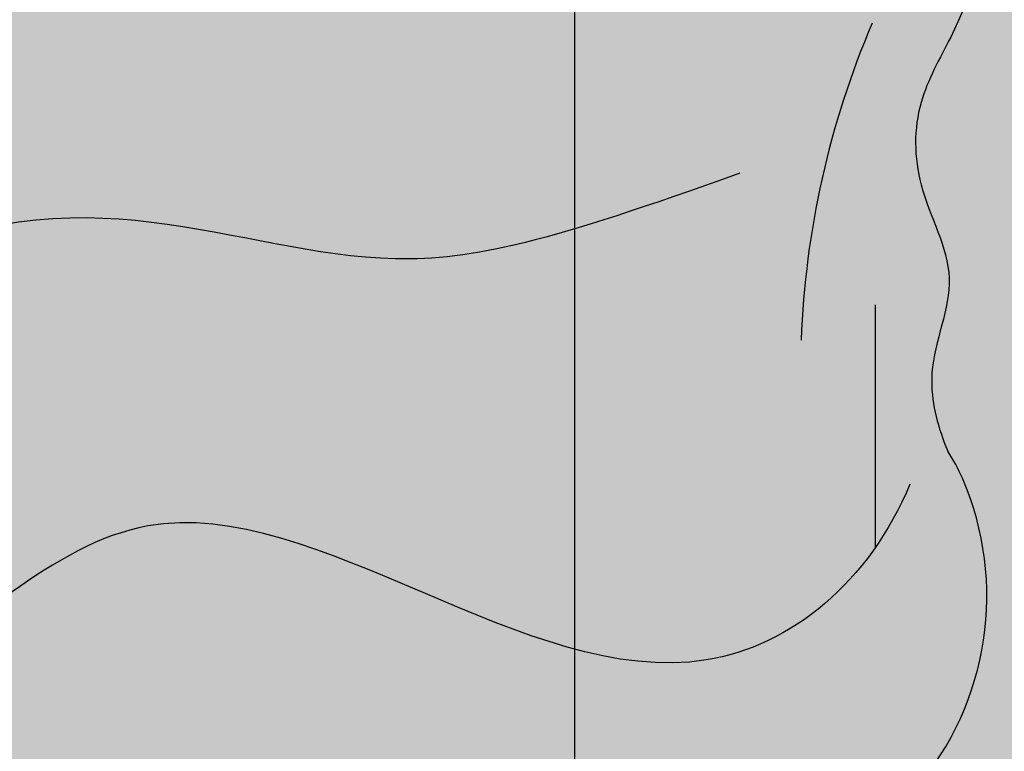
# Model space of a CAD drawing. Units: inches. Extents: x 1704 to 6393, y -157 to 1172.
# Tile 36 of 122: x 2526 to 2564, y 162 to 190. Entities that reach past the tile are written whole.
import ezdxf

# ---------------------------------------------------------------- set-up
doc = ezdxf.new("R2010")
doc.units = ezdxf.units.IN
doc.header["$MEASUREMENT"] = 0
for name, color, linetype, lineweight in [('A-ANNO-DIMS', 7, 'Continuous', 13), ('A-FURN', 8, 'Continuous', 18), ('estofado', 7, 'Continuous', 25)]:
    doc.layers.add(name, color=color, linetype=linetype, lineweight=lineweight)
doc.layers.add('A-FLOR-PATT', color=7, linetype='Continuous', lineweight=13, true_color=0xf2f2f2)
doc.styles.get("Standard").update_dxf_attribs({"font": 'arial.ttf'})
doc.dimstyles.get("Standard").update_dxf_attribs({"dimtxt": 6, "dimasz": 2, "dimexe": 0.18, "dimexo": 0.0625, "dimgap": 0.09, "dimtad": 0, "dimtih": 1, "dimtoh": 1, "dimdec": 1, "dimzin": 0, "dimdsep": 46, "dimlunit": 3, "dimtxsty": 'Standard', "dimblk": 'ARCHTICK', "dimcen": 0.09, "dimadec": 0, "dimazin": 0, "dimtfac": 1, "dimtdec": 1, "dimtofl": 0, "dimtmove": 0, "dimatfit": 3, "dimfxl": 1, "dimtolj": 1, "dimtzin": 0, "dimarcsym": 0})

# ---------------------------------------------------------------- blocks, each defined once
blk = doc.blocks.new('Cama Box Regencia LOLA')
at = {"layer": 'estofado', "ltscale": 0.2}
h = blk.add_hatch(color=256, dxfattribs=at)
h.dxf.hatch_style = 1
h.set_gradient(color1=(206, 178, 131), color2=(233, 221, 200), one_color=1, tint=0.8500000238418579, name='CURVED')
edge = h.paths.add_edge_path()
edge.add_spline(control_points=[(0.9233883396182136, -2.254908822900802), (0.9143712174658276, -2.237158585978875), (0.8971704820246486, -2.20329887728792), (0.9295105801843419, -2.140290914518345), (0.848651568119294, -2.10957861148239), (0.9047062348403186, -2.046222426005954), (0.8299480774321636, -1.990932361540615), (0.9387479200587449, -1.92692496801726), (0.8590435458045249, -1.86767849203585), (0.8322262745575699, -1.826028043643361), (0.8247981799574972, -1.810442049687992)], knot_values=[0, 0, 0, 0, 0.0575832900035364, 0.1098437972159638, 0.1698138218664432, 0.2255174829302509, 0.2824861515521905, 0.3632291183773252, 0.4509842065695901, 0.5012091817853866, 0.5012091817853866, 0.5012091817853866, 0.5012091817853866], degree=3, periodic=0)
edge.add_spline(control_points=[(0.8247981799572698, -1.810442049688447), (0.8512430237993839, -1.769990096378137), (0.8869160776755506, -1.705010622333873), (0.9070359522544322, -1.586338752195842), (0.8536462472426364, -1.488247672851343), (0.8944567470317679, -1.387739666353695), (0.8643796102055603, -1.342420998864781), (0.8547271521993025, -1.327877176513538)], knot_values=[0, 0, 0, 0, 0.1438744691785906, 0.2224893870322766, 0.3492927143212738, 0.4561786976395368, 0.5066917301592304, 0.5066917301592304, 0.5066917301592304, 0.5066917301592304], degree=3, periodic=0)
edge.add_spline(control_points=[(0.8547271521993025, -1.327877176513538), (0.7873766543807506, -1.256744909425322), (0.6449024721503065, -1.106270719748692), (0.3977250465933366, -1.412092721352792), (0.0338148848931041, -1.279726484458706), (-0.3488365122128698, -1.179158668568902), (-0.6188339616464873, -1.25080943574278), (-0.7460155200169539, -1.321708019985464)], knot_values=[0.0991852523588446, 0.0991852523588446, 0.0991852523588446, 0.0991852523588446, 0.3453008654366167, 0.6198216521345741, 0.9826525916749167, 1.386093159660275, 1.810554634340498, 1.810554634340498, 1.810554634340498, 1.810554634340498], degree=3, periodic=0)
edge.add_spline(control_points=[(-0.7460155199962628, -1.32170802000337), (-0.8056354908857201, -1.352141651537124), (-0.8226532004149476, -1.367823298399059), (-0.8348745804664758, -1.38184410903591)], knot_values=[0.0062456970656236, 0.0062456970656236, 0.0062456970656236, 0.0062456970656236, 0.0554759259147193, 0.0554759259147193, 0.0554759259147193, 0.0554759259147193], degree=3, periodic=0)
edge.add_spline(control_points=[(-0.8348745804664758, -1.38184410903591), (-0.8364250716851984, -1.383622888820184), (-0.8378983647115774, -1.385374937005849), (-0.8393716577378427, -1.387126985191514)], knot_values=[0, 0, 0, 0, 0.0062456970656236, 0.0062456970656236, 0.0062456970656236, 0.0062456970656236], degree=3, periodic=0)
edge.add_arc((-0.6180450437709624, -1.576392779500167), 0.2912164331649039, 139.4648411061637, 203.3711573294546)
edge.add_arc((-0.7011750866292914, -1.609837078845487), 0.2016528082906132, 204.0179006417974, 212.6189639884946)
edge.add_spline(control_points=[(-0.8710220093900034, -1.718537943240505), (-0.8696870122217887, -1.721658691442996), (-0.8597709916446092, -1.746046247230935), (-0.8464685798230674, -1.804421032451443), (-0.888988689927828, -1.889951451602371), (-0.8378676506146121, -1.973422824210047), (-0.8371590179440318, -2.05992368952792), (-0.8871569320951948, -2.144598622072578), (-0.908935644436724, -2.210906123939594), (-0.9233883398977695, -2.254908823284267)], knot_values=[0, 0, 0, 0, 0.0101500649009363, 0.0785829584511912, 0.1732273504791735, 0.2688802694005398, 0.3498050162211252, 0.4202002266429896, 0.5590752189863636, 0.5590752189863636, 0.5590752189863636, 0.5590752189863636], degree=3, periodic=0)
edge.add_ellipse((-0.9040800600764669, -2.258882422916315), major_axis=(0.0267880171833212, 0.0267880171833213), ratio=0.4535320972039226, start_angle=94.15910660291303, end_angle=123.37101895145429, ccw=False)
edge.add_ellipse((-0.8772920428931456, -2.232094405732993), major_axis=(0.0772920428927364, 0.0772920428927364), ratio=0.168252450050839, start_angle=-1.0527401173021644e-10, end_angle=156.3071135567154, ccw=False)
edge.add_line((-0.8000000000002955, -2.154802362840428), (0.7999592378284888, -2.154802362840428))
edge.add_arc((0.9462065466516378, -2.098298447668867), 0.1567831871334379, 200.9447658774159, 201.1244713640487, ccw=False)
edge.add_arc((1.115979327553759, -2.004946707326951), 0.3497136727815615, 205.2898146244752, 205.3730108333857)
edge.add_ellipse((0.8772920428930319, -2.232094405732993), major_axis=(-0.0772920428927364, 0.0772920428927364), ratio=0.168252450050839, start_angle=203.6928864432847, end_angle=359.99999999994674, ccw=False)
edge.add_ellipse((0.9040800600763532, -2.258882422916315), major_axis=(-0.0267880171833213, 0.0267880171833213), ratio=0.4535320972039226, start_angle=236.6289810485458, end_angle=265.84089339708703, ccw=False)
blk.add_line((-0.7999999999999546, -1.624303127646271), (-0.7999999999999546, -1.862122701256737), dxfattribs=at)
for centre, radius, start, end in [((-0.618045043771076, -1.576392779500224), 0.2912164331649248, 139.4648411061415, 203.3711573294531), ((-0.7011750866354305, -1.609837078830935), 0.2016528082909061, 204.017900646285, 212.6189640158667), ((-1.599544017339439, -1.795539319485669), 0.8732121282601557, 336.8495239496693, 357.9002538876362)]:
    blk.add_arc(centre, radius, start, end, dxfattribs=at)
for points, knots in [([(-0.8337777191962914, -1.686127396833001), (-0.7936227331957753, -1.590003258421234), (-0.5563859991466416, -1.394748990587913), (-0.1321102153461879, -1.783182047565389), (0.1908245506583626, -1.429131816234075), (0.5373208507353411, -1.424480211867205), (0.720102724937533, -1.549855593291283), (0.836774155394778, -1.71068108627179)], [0.0299011711635954, 0.0299011711635954, 0.0299011711635954, 0.0299011711635954, 0.2769669118207226, 0.7971145189980146, 1.093669199334649, 1.464665995707328, 1.788488893467898, 1.788488893467898, 1.788488893467898, 1.788488893467898]), ([(-0.6667836004502306, -1.991594303623287), (-0.4801926263546648, -1.924290517138388), (-0.2421721137753821, -1.866692280098163), (0.067250899423243, -2.056782250863193), (0.4752270537671848, -1.673138005031375), (0.3282580065483671, -2.063228784622481), (0.6572625331713198, -1.982435509858419)], [0.0299011711635954, 0.0299011711635954, 0.0299011711635954, 0.0299011711635954, 0.2769669118207226, 0.7971145189980146, 1.093669199334649, 1.16835959978728, 1.16835959978728, 1.16835959978728, 1.16835959978728]), ([(-0.9233883398977695, -2.254908823284267), (-0.908935644436724, -2.210906123939594), (-0.8871569320951948, -2.144598622072578), (-0.8371590179440318, -2.05992368952792), (-0.8378676506146121, -1.973422824210047), (-0.888988689927828, -1.889951451602371), (-0.8464685798230674, -1.804421032451443), (-0.8597709916446092, -1.746046247230935), (-0.8696870122217887, -1.721658691442996), (-0.8710220093900034, -1.718537943240505)], [0, 0, 0, 0, 0.1388749923433741, 0.2092702027652384, 0.2901949495858238, 0.3858478685071901, 0.4804922605351724, 0.5489251540854273, 0.5590752189863636, 0.5590752189863636, 0.5590752189863636, 0.5590752189863636])]:
    blk.add_open_spline(points, degree=3, knots=knots, dxfattribs=at)
blk = doc.blocks.new('_ArchTick')
at = {"color": 0, "linetype": 'ByBlock', "const_width": 0.15}
blk.add_lwpolyline([(-0.5, -0.5), (0.5, 0.5)], dxfattribs=at)
blk = doc.blocks.new('*D93')
at = {"layer": 'A-ANNO-DIMS', "color": 0, "lineweight": -2, "transparency": 16777216}
for p, q in [((2605.286074000001, 895.2129740000005), (1829.697551000002, 895.2129740000003)), ((1829.877551000002, 895.2129740000003), (1829.877551000002, 495.8664119263302)), ((1829.877551000002, 90.2129739999999), (1829.877551000002, 489.5595360736699)), ((2605.286074000001, 90.21297400000003), (1829.697551000002, 90.2129739999999))]:
    blk.add_line(p, q, dxfattribs=at)
at = {"layer": 'Defpoints', "color": 0, "lineweight": -3, "transparency": 16777216}
for p in [(2605.348574000001, 895.2129740000005), (1829.877551000002, 90.2129739999999), (2605.348574000001, 90.21297400000003)]:
    blk.add_point(p, dxfattribs=at)
at = {"layer": 'A-ANNO-DIMS', "color": 0, "lineweight": -2, "transparency": 16777216, "xscale": 2, "yscale": 2, "zscale": 2}
for p, rotation in [((1829.877551000002, 895.2129740000003), 90), ((1829.877551000002, 90.2129739999999), 270)]:
    blk.add_blockref('_ArchTick', p, dxfattribs=dict(at, rotation=rotation))
at = {"layer": 'A-ANNO-DIMS', "color": 0, "transparency": 16777216, "insert": (1829.877551000001, 492.7129739999994), "char_height": 6, "attachment_point": 5}
blk.add_mtext('\\A1;805', dxfattribs=at)
blk = doc.blocks.new('*D105')
at = {"layer": 'A-ANNO-DIMS', "color": 0, "lineweight": -2, "transparency": 16777216}
for p, q in [((2451.737975, 615.150474), (2451.737975, -64.9670259999999)), ((2547.348574, 615.150474), (2547.348574, -64.9670259999999)), ((2451.737975, -64.787026), (2489.908936164393, -64.787026)), ((2547.348574, -64.787026), (2509.177612835607, -64.787026))]:
    blk.add_line(p, q, dxfattribs=at)
at = {"layer": 'Defpoints', "color": 0, "lineweight": -3, "transparency": 16777216}
for p in [(2451.737975, 615.212974), (2547.348574, 615.212974), (2547.348574, -64.787026)]:
    blk.add_point(p, dxfattribs=at)
at = {"layer": 'A-ANNO-DIMS', "color": 0, "lineweight": -2, "transparency": 16777216, "xscale": 2, "yscale": 2, "zscale": 2, "rotation": 180}
blk.add_blockref('_ArchTick', (2451.737975, -64.787026), dxfattribs=at)
at = {"layer": 'A-ANNO-DIMS', "color": 0, "lineweight": -2, "transparency": 16777216, "xscale": 2, "yscale": 2, "zscale": 2}
blk.add_blockref('_ArchTick', (2547.348574, -64.787026), dxfattribs=at)
at = {"layer": 'A-ANNO-DIMS', "color": 0, "transparency": 16777216, "insert": (2499.5432745, -64.787026), "char_height": 6, "attachment_point": 5}
blk.add_mtext('\\A1;95.61', dxfattribs=at)

msp = doc.modelspace()

# ---------------------------------------------------------------- hatches: boundary and pattern name
at = {"layer": 'A-FLOR-PATT', "transparency": 33554528}
h = msp.add_hatch(color=256, dxfattribs=at)
h.dxf.hatch_style = 1
h.paths.add_polyline_path([(2325.348574056059, 863.2129735309796), (2325.348574056059, 887.2129735309796), (2263.348574056059, 887.2129735309796), (2167.348574056059, 887.2129735309794), (2081.348574056061, 887.2129735309792), (2081.348574056061, 719.2129735309785), (2277.348574056059, 719.2129735309787), (2277.348574056059, 711.2129735309788), (2277.348574056059, 372.212973530979), (2349.348574056059, 372.212973530979), (2381.348574056059, 372.2129735309789), (2381.348574056059, 364.2129735309789), (2353.348574056059, 364.2129735309789), (2353.348574056059, 270.2129735309788), (2381.348574056059, 270.2129735309788), (2381.348574056059, 266.2129735309788), (2357.348574056059, 266.2129735309788), (2357.348574056059, 98.21297353097884), (2381.348574056059, 98.21297353097897), (2385.181056550604, 98.21297353097884), (2386.482186711948, 98.21297353097884), (2424.21496140017, 98.21297353097884), (2425.516091561514, 98.21297353097884), (2429.348574056059, 98.21297353097897), (2597.348574056059, 98.21297353097884), (2597.348574056059, 146.2129735309788), (2597.348574056059, 218.2129735309788), (2597.348574056059, 266.2129735309788), (2423.348574056059, 266.2129735309788), (2423.348574056059, 270.2129735309788), (2473.348574056059, 270.2129735309788), (2473.348574056059, 294.2129735309789), (2477.348574056059, 294.2129735309789), (2477.348574056059, 270.2129735309788), (2547.348574056059, 270.2129735309788), (2547.348574056059, 364.2129735309788), (2477.348574056059, 364.2129735309788), (2477.348574056059, 318.2129735309788), (2473.348574056059, 318.2129735309787), (2473.348574056059, 364.2129735309789), (2423.348574056059, 364.2129735309788), (2423.348574056059, 372.2129735309788), (2469.348574056059, 372.2129735309788), (2469.348574056059, 459.2129735309789), (2469.348574056059, 538.2129735309788), (2350.348574056059, 538.2129735309788), (2350.348574056059, 565.7129735309788), (2358.348574056059, 565.7129735309788), (2358.348574056059, 545.2129735309788), (2420.348574056059, 545.2129735309788), (2420.348574056059, 610.2129735309788), (2358.348574056059, 610.2129735309788), (2358.348574056059, 589.7129735309788), (2350.348574056059, 589.7129735309788), (2350.348574056059, 615.2129735309788), (2425.348574056059, 615.2129735309788), (2425.348574056059, 607.2129735309788), (2425.348574056059, 546.2129735309788), (2469.348574056059, 546.2129735309788), (2514.34857405606, 546.212973530979), (2514.34857405606, 607.2129735309788), (2449.348574056059, 607.2129735309788), (2449.348574056059, 615.2129735309788), (2451.737974987759, 615.2129735309788), (2451.737974987759, 659.2129735309788), (2427.737974987759, 659.2129735309788), (2427.737974987759, 665.2129735309788), (2367.737974987758, 665.2129735309788), (2367.737974987758, 667.2129735309788), (2367.737974987758, 711.2129735309788), (2325.348574056059, 711.2129735309788), (2325.348574056059, 719.2129735309785), (2325.348574056059, 755.2129735309787), (2325.348574056059, 763.2129735309788)])
h.paths.add_polyline_path([(2233.85817000392, 822.532660166629, -0.1872470486944155), (2233.85817000392, 809.1396667958562), (2231.697030374885, 808.8044951349628, 0.0848927708004382), (2233.130501812631, 814.4858417746204), (2230.423974436808, 814.4858417746204, -0.1042581087707907), (2228.553363812687, 808.3129425443484), (2217.750790159711, 807.1555239386723, -0.2222222222222219), (2217.750790159711, 824.5168030238124), (2228.553363812687, 823.3593844181363, -0.1042581087707933), (2230.423974436808, 817.1864851878643), (2233.130501812631, 817.1864851878643, 0.08489277080044), (2231.697030374885, 822.8678318275219)], flags=16)
h.paths.add_polyline_path([(2213.621360876743, 833.1974425663823), (2213.621360876743, 798.4748843961024), (2156.047684459484, 798.4748843961034), (2156.047684459485, 833.1974425663813)], flags=16)
h.paths.add_polyline_path([(2203.931929661768, 848.0987249710489), (2205.089348267444, 837.2961513180724, -0.2222222222222264), (2187.728069182304, 837.2961513180724), (2188.88548778798, 848.0987249710485, -0.104258108770792), (2195.058387018252, 849.9693355951691), (2195.058387018252, 852.6758629709927, 0.084892770800438), (2189.377040378595, 851.2423915332469), (2189.712212039488, 853.4035311622828, -0.1872470486944166), (2203.105205410261, 853.4035311622828), (2203.440377071154, 851.2423915332469, 0.084892770800438), (2197.759030431496, 852.6758629709927), (2197.759030431496, 849.9693355951691, -0.1042581087707896)], flags=16)
h.paths.add_polyline_path([(2181.940976153924, 837.2961513180726, -0.2222222222222323), (2164.579697068783, 837.2961513180724), (2165.73711567446, 848.0987249710487, -0.1042581087707905), (2171.910014904732, 849.9693355951691), (2171.910014904732, 852.6758629709927, 0.0848927708004445), (2166.228668265074, 851.2423915332469), (2166.563839925967, 853.403531162283, -0.1872470486944096), (2179.95683329674, 853.4035311622828), (2180.292004957633, 851.2423915332465, 0.0848927708004458), (2174.610658317976, 852.6758629709927), (2174.610658317976, 849.9693355951691, -0.104258108770801), (2180.783557548248, 848.0987249710482)], flags=16)
h.paths.add_polyline_path([(2205.089348267444, 794.376175644412), (2203.931929661768, 783.5736019914364, -0.1042581087707934), (2197.759030431496, 781.7029913673155), (2197.759030431496, 778.9964639914921, 0.084892770800439), (2203.440377071154, 780.4299354292382), (2203.105205410261, 778.2687958002022, -0.1872470486944172), (2189.712212039488, 778.2687958002018), (2189.377040378595, 780.4299354292377, 0.0848927708004369), (2195.058387018252, 778.9964639914919), (2195.058387018252, 781.7029913673153, -0.1042581087707904), (2188.88548778798, 783.5736019914358), (2187.728069182304, 794.3761756444126, -0.2222222222222231)], flags=16)
h.paths.add_polyline_path([(2181.940976153924, 794.376175644412), (2180.783557548248, 783.5736019914364, -0.1042581087708008), (2174.610658317976, 781.7029913673153), (2174.610658317976, 778.9964639914921, 0.0848927708004458), (2180.292004957633, 780.4299354292382), (2179.95683329674, 778.268795800202, -0.1872470486944096), (2166.563839925967, 778.2687958002018), (2166.228668265074, 780.4299354292378, 0.0848927708004446), (2171.910014904732, 778.9964639914919), (2171.910014904732, 781.7029913673153, -0.1042581087707904), (2165.73711567446, 783.5736019914358), (2164.579697068783, 794.3761756444123, -0.2222222222222294)], flags=16)
h.paths.add_polyline_path([(2151.918255176517, 807.1555239386723), (2141.115681523541, 808.3129425443484, -0.1042581087707911), (2139.24507089942, 814.4858417746204), (2136.538543523597, 814.4858417746204, 0.08489277080044), (2137.972014961343, 808.8044951349626), (2135.810875332307, 809.1396667958562, -0.1872470486944109), (2135.810875332307, 822.5326601666285), (2137.972014961343, 822.8678318275221, 0.0848927708004416), (2136.538543523597, 817.1864851878643), (2139.24507089942, 817.1864851878643, -0.104258108770793), (2141.115681523541, 823.3593844181363), (2151.918255176517, 824.5168030238124, -0.2222222222222205)], flags=16)
h.paths.add_polyline_path([(2357.868011454448, 363.4102250290031), (2358.813881560335, 363.4102250290031, 0.7537604849588476)], flags=16)
h.paths.add_polyline_path([(2372.241054283868, 363.1167008961685), (2372.248110816919, 363.1167008961685), (2372.248110816919, 363.3425764997267), (2371.30224071103, 363.3425764997267), (2371.30224071103, 363.1392706554335, -1.360391292333951)], flags=16)
h.paths.add_polyline_path([(2371.309297244092, 272.7157694655011), (2371.30224071103, 272.7157694655011), (2371.30224071103, 272.4898938619428), (2372.248110816919, 272.4898938619428), (2372.248110816919, 272.6931997062759, -1.360391292393621)], flags=16)
h.paths.add_polyline_path([(2357.875067987504, 272.7157694655011), (2357.868011454452, 272.7157694655011), (2357.868011454452, 272.4898938619428), (2358.813881560341, 272.4898938619428), (2358.813881560341, 272.6931997062361, -1.360391292333948)], flags=16)
h.paths.add_polyline_path([(2353.768696905258, 363.0736921025416), (2376.347425366111, 363.0736921025416), (2376.347425366111, 272.7587782591281), (2353.768696905258, 272.7587782591281)], flags=16)
h.paths.add_polyline_path([(2354.772195947961, 362.0701930598379), (2375.343926323407, 362.0701930598379), (2375.343926323407, 273.7622773018316), (2354.772195947961, 273.7622773018318)], flags=0)
h.paths.add_polyline_path([(2357.868011454452, 363.3425764997267), (2358.813881560341, 363.3425764997266), (2358.813881560341, 363.1167008961684), (2357.868011454452, 363.1167008961684)], flags=16)
h.paths.add_polyline_path([(2359.287941640134, 359.1843485433627), (2359.287941640134, 360.0631949744305), (2370.828180631237, 360.0631949744362), (2370.828180631237, 359.1843485433769), (2374.332057422314, 359.1843485433812), (2374.332057422312, 358.4635369582513), (2372.835178716611, 358.4635369582524), (2372.835178716611, 357.5410357047662), (2374.332057422314, 357.5410357047678), (2374.332057422312, 356.8202241196381), (2372.835178716611, 356.820224119639), (2372.835178716611, 355.897722866153), (2374.332057422314, 355.8977228661546), (2374.332057422312, 355.1769112810248), (2372.835178716611, 355.1769112810259), (2372.835178716611, 354.2544100275397), (2374.332057422334, 354.2544100275415), (2374.332057422331, 353.5335984424117), (2372.835178716631, 353.5335984424126), (2372.835178716631, 352.6110971889265), (2374.332057422334, 352.6110971889282), (2374.332057422331, 351.8902856037984), (2372.835178716631, 351.8902856037993), (2372.835178716631, 350.9677843503132), (2374.332057422334, 350.967784350315), (2374.332057422331, 350.2469727651852), (2372.835178716631, 350.2469727651861), (2372.835178716631, 349.3244715117), (2374.332057422334, 349.3244715117017), (2374.332057422331, 348.603659926572), (2372.835178716631, 348.6036599265729), (2372.835178716631, 347.6811586730868), (2374.332057422334, 347.6811586730886), (2374.332057422331, 346.9603470879587), (2372.835178716631, 346.9603470879598), (2372.835178716631, 346.0378458344735), (2374.332057422334, 346.0378458344753), (2374.332057422331, 345.3170342493456), (2372.835178716631, 345.3170342493465), (2372.835178716631, 344.3945329958605), (2374.332057422334, 344.3945329958621), (2374.332057422331, 343.6737214107324), (2372.835178716631, 343.6737214107334), (2372.835178716631, 342.751220157247), (2374.332057422334, 342.7512201572489), (2374.332057422331, 342.0304085721191), (2372.835178716631, 342.03040857212), (2372.835178716631, 341.1079073186338), (2374.332057422334, 341.1079073186356), (2374.332057422331, 340.3870957335057), (2372.835178716631, 340.3870957335066), (2372.835178716631, 339.4645944800207), (2374.332057422334, 339.4645944800223), (2374.332057422331, 338.7437828948924), (2372.835178716648, 338.7437828948933), (2372.835178716648, 337.8212816414076), (2374.332057422334, 337.8212816414093), (2374.332057422331, 337.1004700562794), (2372.835178716648, 337.1004700562803), (2372.835178716648, 336.1779688027942), (2374.332057422334, 336.1779688027961), (2374.332057422331, 335.4571572176662), (2372.835178716648, 335.4571572176673), (2372.835178716648, 334.5346559641809), (2374.332057422334, 334.5346559641828), (2374.332057422331, 333.8138443790529), (2372.835178716648, 333.8138443790539), (2372.835178716648, 332.8913431255679), (2374.332057422334, 332.8913431255696), (2374.332057422331, 332.1705315404397), (2372.835178716648, 332.1705315404406), (2372.835178716648, 331.2480302869545), (2374.332057422334, 331.2480302869563), (2374.332057422331, 330.5272187018265), (2372.835178716648, 330.5272187018273), (2372.835178716648, 329.6047174483413), (2374.332057422334, 329.6047174483431), (2374.332057422331, 328.8839058632133), (2372.835178716648, 328.8839058632143), (2372.835178716648, 327.9614046097282), (2374.332057422334, 327.9614046097298), (2374.332057422331, 327.2405930246), (2372.835178716648, 327.2405930246009), (2372.835178716648, 326.3180917711149), (2374.332057422334, 326.3180917711167), (2374.332057422331, 325.5972801859869), (2372.835178716648, 325.5972801859877), (2372.835178716648, 324.6747789325016), (2374.332057422334, 324.6747789325034), (2374.332057422331, 323.9539673473736), (2372.835178716648, 323.9539673473746), (2372.835178716648, 323.0314660938884), (2374.332057422334, 323.0314660938901), (2374.332057422331, 322.3106545087603), (2372.835178716648, 322.3106545087613), (2372.835178716648, 321.3881532552753), (2374.332057422334, 321.388153255277), (2374.332057422331, 320.6673416701471), (2372.835178716648, 320.6673416701481), (2372.835178716648, 319.7448404166621), (2374.332057422334, 319.7448404166638), (2374.332057422331, 319.0240288315339), (2372.835178716648, 319.0240288315348), (2372.835178716648, 318.1015275780487), (2374.332057422334, 318.1015275780504), (2374.332057422331, 317.3807159929205), (2372.835178716648, 317.3807159929214), (2372.835178716648, 316.4582147394357), (2374.332057422334, 316.4582147394373), (2374.332057422331, 315.7374031543073), (2372.835178716648, 315.7374031543084), (2372.835178716648, 314.8149019008223), (2374.332057422334, 314.8149019008241), (2374.332057422331, 314.0940903156943), (2372.835178716648, 314.0940903156952), (2372.835178716648, 313.171589062209), (2374.332057422334, 313.1715890622108), (2374.332057422331, 312.450777477081), (2372.835178716648, 312.4507774770819), (2372.835178716648, 311.5282762235959), (2374.332057422334, 311.5282762235977), (2374.332057422331, 310.8074646384678), (2372.835178716648, 310.8074646384687), (2372.835178716648, 309.8849633849827), (2374.332057422334, 309.8849633849844), (2374.332057422331, 309.1641517998546), (2372.835178716648, 309.1641517998555), (2372.835178716648, 308.2416505463693), (2374.332057422334, 308.2416505463712), (2374.332057422331, 307.5208389612412), (2372.835178716648, 307.5208389612421), (2372.835178716648, 306.5983377077562), (2374.332057422334, 306.598337707758), (2374.332057422331, 305.8775261226281), (2372.835178716648, 305.8775261226289), (2372.835178716648, 304.955024869143), (2374.332057422334, 304.9550248691447), (2374.332057422331, 304.2342132840149), (2372.835178716648, 304.2342132840158), (2372.835178716648, 303.3117120305298), (2374.332057422334, 303.3117120305316), (2374.332057422331, 302.5909004454018), (2372.835178716648, 302.5909004454027), (2372.835178716648, 301.6683991919165), (2374.332057422334, 301.6683991919183), (2374.332057422331, 300.9475876067885), (2372.835178716648, 300.9475876067894), (2372.835178716648, 300.0250863533033), (2374.332057422334, 300.025086353305), (2374.332057422331, 299.3042747681752), (2372.835178716648, 299.3042747681761), (2372.835178716648, 298.3817735146902), (2374.332057422334, 298.3817735146919), (2374.332057422331, 297.6609619295621), (2372.835178716648, 297.6609619295629), (2372.835178716648, 296.7384606760769), (2374.332057422334, 296.7384606760786), (2374.332057422331, 296.0176490909488), (2372.835178716648, 296.0176490909498), (2372.835178716648, 295.0951478374636), (2374.332057422334, 295.0951478374653), (2374.332057422331, 294.3743362523355), (2372.835178716648, 294.3743362523364), (2372.835178716648, 293.4518349988504), (2374.332057422334, 293.4518349988522), (2374.332057422331, 292.7310234137224), (2372.835178716648, 292.7310234137233), (2372.835178716648, 291.8085221602371), (2374.332057422334, 291.8085221602389), (2374.332057422331, 291.0877105751091), (2372.835178716648, 291.08771057511), (2372.835178716648, 290.165209321624), (2374.332057422334, 290.1652093216256), (2374.332057422331, 289.4443977364957), (2372.835178716648, 289.4443977364966), (2372.835178716648, 288.5218964830108), (2374.332057422334, 288.5218964830125), (2374.332057422331, 287.8010848978827), (2372.835178716648, 287.8010848978836), (2372.835178716648, 286.8785836443975), (2374.332057422334, 286.8785836443993), (2374.332057422331, 286.1577720592695), (2372.835178716648, 286.1577720592703), (2372.835178716648, 285.2352708057842), (2374.332057422334, 285.2352708057861), (2374.332057422331, 284.5144592206562), (2372.835178716648, 284.514459220657), (2372.835178716648, 283.5919579671712), (2374.332057422334, 283.5919579671728), (2374.332057422331, 282.871146382043), (2372.835178716648, 282.8711463820439), (2372.835178716648, 281.9486451285579), (2374.332057422334, 281.9486451285596), (2374.332057422331, 281.2278335434298), (2372.835178716648, 281.2278335434307), (2372.835178716648, 280.3053322899446), (2374.332057422334, 280.3053322899464), (2374.332057422331, 279.5845207048164), (2372.835178716648, 279.5845207048174), (2372.835178716648, 278.6620194513314), (2374.332057422334, 278.6620194513331), (2374.332057422331, 277.9412078662033), (2372.835178716648, 277.9412078662043), (2372.835178716648, 277.0187066127184), (2374.332057422334, 277.0187066127201), (2374.332057422331, 276.29789502759), (2370.828180631244, 276.2978950275922), (2370.828180631244, 275.7692753872335), (2359.287941640128, 275.7692753872392), (2359.287941640128, 276.2978950275993), (2355.784064849037, 276.2978950276015), (2355.784064849037, 277.0187066126971), (2357.280943554723, 277.0187066126989), (2357.280943554723, 277.9412078662137), (2355.784064849037, 277.9412078662145), (2355.784064849037, 278.6620194513103), (2357.280943554723, 278.6620194513122), (2357.280943554723, 279.5845207048271), (2355.784064849037, 279.584520704828), (2355.784064849037, 280.3053322899236), (2357.280943554723, 280.3053322899253), (2357.280943554723, 281.2278335434403), (2355.784064849037, 281.2278335434412), (2355.784064849037, 281.9486451285369), (2357.280943554723, 281.9486451285387), (2357.280943554723, 282.8711463820535), (2355.784064849037, 282.8711463820543), (2355.784064849037, 283.5919579671501), (2357.280943554723, 283.591957967152), (2357.280943554723, 284.5144592206668), (2355.784064849037, 284.5144592206676), (2355.784064849037, 285.2352708057632), (2357.280943554723, 285.2352708057651), (2357.280943554723, 286.1577720592801), (2355.784064849037, 286.1577720592809), (2355.784064849037, 286.8785836443766), (2357.280943554723, 286.8785836443784), (2357.280943554723, 287.8010848978931), (2355.784064849037, 287.8010848978941), (2355.784064849037, 288.5218964829895), (2357.280943554723, 288.5218964829913), (2357.280943554723, 289.4443977365064), (2355.784064849037, 289.4443977365072), (2355.784064849037, 290.1652093216029), (2357.280943554723, 290.1652093216047), (2357.280943554723, 291.0877105751197), (2355.784064849037, 291.0877105751206), (2355.784064849037, 291.8085221602161), (2357.280943554723, 291.8085221602179), (2357.280943554723, 292.7310234137328), (2355.784064849037, 292.7310234137337), (2355.784064849037, 293.4518349988293), (2357.280943554723, 293.451834998831), (2357.280943554723, 294.3743362523461), (2355.784064849037, 294.3743362523469), (2355.784064849037, 295.0951478374426), (2357.280943554723, 295.0951478374445), (2357.280943554723, 296.0176490909594), (2355.784064849037, 296.0176490909601), (2355.784064849037, 296.7384606760557), (2357.280943554723, 296.7384606760575), (2357.280943554723, 297.6609619295724), (2355.784064849037, 297.6609619295734), (2355.784064849037, 298.3817735146691), (2357.280943554723, 298.3817735146709), (2357.280943554723, 299.3042747681858), (2355.784064849037, 299.3042747681866), (2355.784064849037, 300.0250863532823), (2357.280943554723, 300.0250863532841), (2357.280943554723, 300.9475876067989), (2355.784064849037, 300.9475876067997), (2355.784064849037, 301.6683991918954), (2357.280943554723, 301.6683991918973), (2357.280943554723, 302.5909004454123), (2355.784064849037, 302.5909004454133), (2355.784064849037, 303.3117120305088), (2357.280943554723, 303.3117120305105), (2357.280943554723, 304.2342132840254), (2355.784064849037, 304.2342132840262), (2355.784064849037, 304.9550248691219), (2357.280943554723, 304.9550248691238), (2357.280943554723, 305.8775261226386), (2355.784064849037, 305.8775261226394), (2355.784064849037, 306.5983377077352), (2357.280943554723, 306.5983377077369), (2357.280943554723, 307.5208389612518), (2355.784064849037, 307.5208389612528), (2355.784064849037, 308.2416505463484), (2357.280943554723, 308.2416505463501), (2357.280943554723, 309.1641517998652), (2355.784064849037, 309.1641517998661), (2355.784064849037, 309.8849633849617), (2357.280943554723, 309.8849633849634), (2357.280943554723, 310.8074646384782), (2355.784064849037, 310.8074646384791), (2355.784064849037, 311.5282762235748), (2357.280943554723, 311.5282762235767), (2357.280943554723, 312.4507774770916), (2355.784064849037, 312.4507774770925), (2355.784064849037, 313.171589062188), (2357.280943554723, 313.1715890621898), (2357.280943554723, 314.0940903157049), (2355.784064849037, 314.0940903157058), (2355.784064849037, 314.8149019008013), (2357.280943554723, 314.8149019008032), (2357.280943554723, 315.7374031543179), (2355.784064849037, 315.7374031543187), (2355.784064849037, 316.4582147394146), (2357.280943554723, 316.4582147394165), (2357.280943554723, 317.3807159929311), (2355.784064849037, 317.3807159929321), (2355.784064849037, 318.1015275780277), (2357.280943554723, 318.1015275780295), (2357.280943554723, 319.0240288315445), (2355.784064849037, 319.0240288315454), (2355.784064849037, 319.744840416641), (2357.280943554723, 319.7448404166428), (2357.280943554723, 320.6673416701576), (2355.784064849037, 320.6673416701585), (2355.784064849037, 321.3881532552541), (2357.280943554723, 321.388153255256), (2357.280943554723, 322.3106545087708), (2355.784064849037, 322.3106545087718), (2355.784064849037, 323.0314660938674), (2357.280943554723, 323.0314660938692), (2357.280943554723, 323.9539673473843), (2355.784064849037, 323.9539673473851), (2355.784064849037, 324.6747789324806), (2357.280943554723, 324.6747789324824), (2357.280943554723, 325.5972801859974), (2355.784064849037, 325.5972801859983), (2355.784064849037, 326.3180917710939), (2357.280943554723, 326.3180917710958), (2357.280943554723, 327.2405930246105), (2355.784064849037, 327.2405930246113), (2355.784064849037, 327.9614046097071), (2357.280943554723, 327.961404609709), (2357.280943554723, 328.8839058632238), (2355.784064849037, 328.8839058632245), (2355.784064849037, 329.6047174483202), (2357.280943554723, 329.604717448322), (2357.280943554723, 330.527218701837), (2355.784064849037, 330.5272187018379), (2355.784064849037, 331.2480302869335), (2357.280943554723, 331.2480302869353), (2357.280943554723, 332.1705315404502), (2355.784064849037, 332.170531540451), (2355.784064849037, 332.8913431255468), (2357.280943554723, 332.8913431255486), (2357.280943554723, 333.8138443790634), (2355.784064849037, 333.8138443790642), (2355.784064849037, 334.5346559641599), (2357.280943554723, 334.5346559641618), (2357.280943554723, 335.4571572176767), (2355.784064849037, 335.4571572176776), (2355.784064849037, 336.1779688027732), (2357.280943554723, 336.177968802775), (2357.280943554723, 337.1004700562898), (2355.784064849037, 337.1004700562908), (2355.784064849037, 337.8212816413864), (2357.280943554723, 337.8212816413883), (2357.280943554723, 338.7437828949031), (2355.784064849037, 338.743782894904), (2355.784064849037, 339.4645944799996), (2357.280943554706, 339.4645944800013), (2357.280943554706, 340.3870957335163), (2355.784064849037, 340.3870957335173), (2355.784064849037, 341.1079073186129), (2357.280943554706, 341.1079073186146), (2357.280943554706, 342.0304085721296), (2355.784064849037, 342.0304085721304), (2355.784064849037, 342.7512201572262), (2357.280943554706, 342.751220157228), (2357.280943554706, 343.6737214107429), (2355.784064849037, 343.6737214107437), (2355.784064849037, 344.3945329958394), (2357.280943554706, 344.3945329958412), (2357.280943554706, 345.317034249356), (2355.784064849037, 345.3170342493569), (2355.784064849037, 346.0378458344526), (2357.280943554706, 346.0378458344544), (2357.280943554706, 346.9603470879692), (2355.784064849037, 346.9603470879701), (2355.784064849037, 347.6811586730658), (2357.280943554706, 347.6811586730677), (2357.280943554706, 348.6036599265824), (2355.784064849037, 348.6036599265833), (2355.784064849037, 349.324471511679), (2357.280943554706, 349.3244715116809), (2357.280943554706, 350.2469727651956), (2355.784064849037, 350.2469727651966), (2355.784064849037, 350.9677843502922), (2357.280943554706, 350.9677843502939), (2357.280943554706, 351.8902856038089), (2355.784064849037, 351.8902856038098), (2355.784064849037, 352.6110971889055), (2357.280943554706, 352.6110971889072), (2357.280943554706, 353.5335984424222), (2355.784064849037, 353.533598442423), (2355.784064849037, 354.2544100275187), (2357.280943554686, 354.2544100275204), (2357.280943554686, 355.1769112810354), (2355.784064849017, 355.1769112810362), (2355.784064849017, 355.897722866132), (2357.280943554686, 355.8977228661338), (2357.280943554686, 356.8202241196486), (2355.784064849017, 356.8202241196495), (2355.784064849017, 357.5410357047453), (2357.280943554686, 357.5410357047471), (2357.280943554686, 358.4635369582618), (2355.784064849017, 358.4635369582626), (2355.784064849017, 359.1843485433584)], flags=0)

# ---------------------------------------------------------------- block references
at = {"layer": 'A-FURN', "xscale": 39.22313671019584, "yscale": 39.22313671019584, "zscale": 39.22313671019584, "rotation": 180}
msp.add_blockref('Cama Box Regencia LOLA', (2527.569415053021, 106.0625493409584), dxfattribs=at)

# ---------------------------------------------------------------- dimensions: what is measured, and where the dimension line sits
at = {"layer": 'A-ANNO-DIMS'}
dim = msp.add_linear_dim(base=(1829.877551000002, 90.2129739999999), p1=(2605.348574000001, 895.212974), p2=(2605.348574000001, 90.21297399999999), angle=90, dimstyle='Standard', override={"dimdec": 0, "dimlfac": 1, "dimrnd": 0, "dimzin": 0, "dimdsep": 46, "dimlunit": 2}, dxfattribs=at)
dim.commit()
dim.dimension.update_dxf_attribs({"geometry": '*D93', "text_midpoint": (1829.877551000001, 492.7129739999994)})
dim = msp.add_linear_dim(base=(2547.348574, -64.787026), p1=(2451.737975, 615.212974), p2=(2547.348574, 615.212974), dimstyle='Standard', override={"dimdec": 2, "dimlfac": 1, "dimrnd": 0, "dimzin": 0, "dimdsep": 46, "dimlunit": 2}, dxfattribs=at)
dim.commit()
dim.dimension.update_dxf_attribs({"geometry": '*D105', "text_midpoint": (2499.5432745, -64.787026)})

doc.saveas('drawing.dxf')
